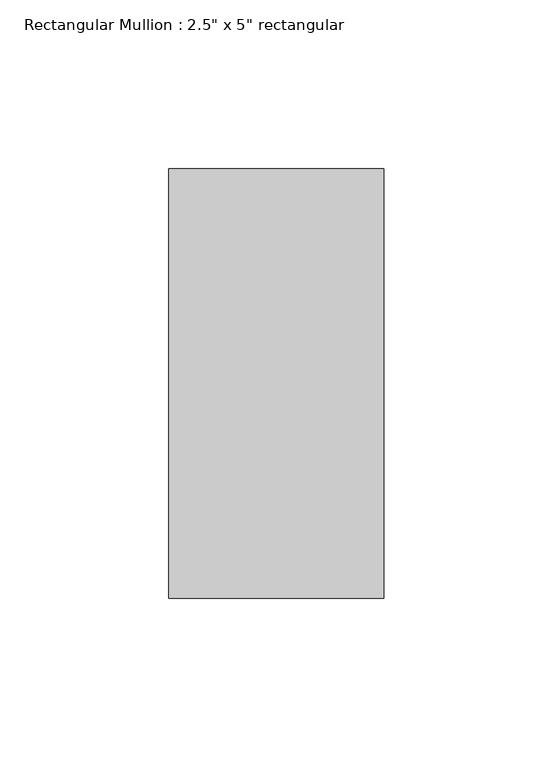
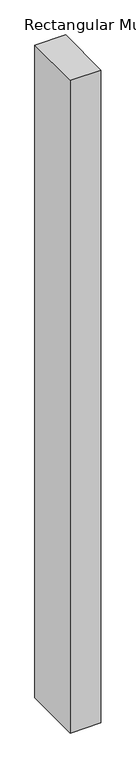
"""IFC4 building model written with IfcOpenShell, lengths in millimetres: member geometry."""

from ifc_helpers import new_model, si_unit, frame, origin, place, context, project, spatial, polyline, outline, extrude, source, transform, mapped, element, save


def member_358e2bc9(model_context):
    return source(origin(), model_context, "Body", "SweptSolid", [
        extrude(outline(polyline([(0.0, 63.5), (0.0, -63.5), (-63.5, -63.5), (-63.5, 63.5), (0.0, 63.5)])), frame((0.0, 0.0, -1431.1740318), z_axis=(0.0, 0.0, 1.0), x_axis=(1.0, 0.0, 0.0)), (0.0, 0.0, 1.0), 1431.1740318),
    ])


if __name__ == "__main__":
    model = new_model("IFC4")
    model_context = context("Model", 3, world=origin())
    ifc_project = project(units=[si_unit("LENGTHUNIT", "METRE", prefix="MILLI")], contexts=[model_context])
    site = spatial("IfcSite", under=ifc_project)
    building = spatial("IfcBuilding", under=site)
    placement = place(None, origin())
    member_shape = member_358e2bc9(model_context)
    element("IfcMember", 1, ObjectType="Rectangular Mullion : 2.5\" x 5\" rectangular", at=placement, inside=building, context=model_context, shape_type="MappedRepresentation", body=[
        mapped(member_shape, transform((0.0, 0.0, 0.0), x_axis=(1.0, 0.0, 0.0), y_axis=(0.0, 1.0, 0.0), z_axis=(0.0, 0.0, 1.0))),
    ])
    save(model, "model.ifc")

# Revit data of these elements
# Type "Rectangular Mullion : 2.5\" x 5\" rectangular"
#   built-in parameter 1007304 = 0.416667 (stored number, unit not read)
#   built-in parameter 1007301 = 0.104167 (stored number, unit not read)
#   built-in parameter 1007300 = 0.104167 (stored number, unit not read)
# Element 1 (IfcMember, "Rectangular Mullion : 2.5\" x 5\" rectangular")
#   Materials on its faces: "Aluminum"
# Materials
#   "Aluminum": class "Metal", colour RGB 247 247 247, transparency 0, Description = "Aluminum 6061", Cost = 0
